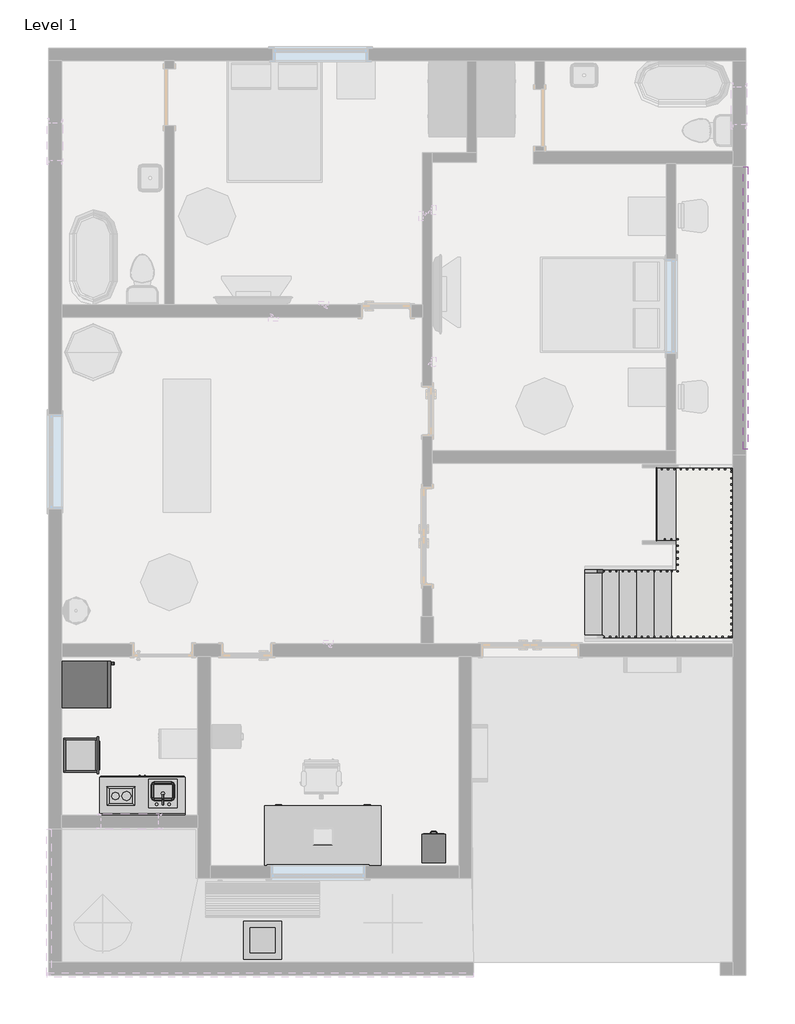
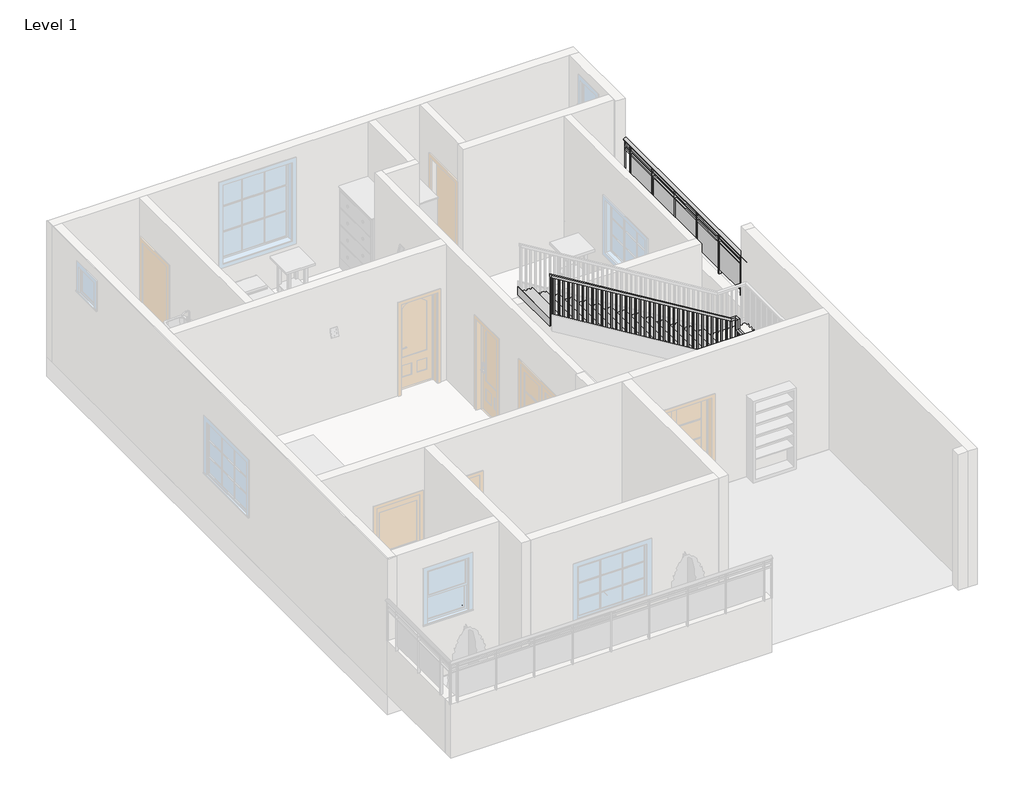
# One storey, part 3 of 4: 4 furniture elements, 4 proxies, 2 railings, 2 stair flights, 1 flow terminal, 1 slab.
"""IFC4 building model written with IfcOpenShell, lengths in millimetres."""

from ifc_helpers import new_model, si_unit, point, frame, origin, place, context, project, spatial, polyline, ellipse_curve, trimmed, outline, extrude, faceted_brep, transform, mapped, element, save
from ifc_brep_helpers import plane_surface, extruded_surface, advanced_brep
from components import proxy_fe84b772, proxy_844211aa, proxy_8b8c2dc4, proxy_a13a33b2, flow_terminal_871c2e40, furniture_d4d3357e, furniture_95afb093, furniture_2fc54265, furniture_b5c51a22, non_monolithic_landing_4509e35c, stair_flight_239b6ec8, stair_flight_7a186021

model = new_model("IFC4")

# Units and contexts
model_context = context("Model", 3, world=origin())
ifc_project = project(units=[si_unit("LENGTHUNIT", "METRE", prefix="MILLI")], contexts=[model_context])

# Site, building, storey
site = spatial("IfcSite", under=ifc_project)
building = spatial("IfcBuilding", under=site)
storey = spatial("IfcBuildingStorey", under=building, Name="Level 1", Elevation=0.0)

# Proxies
placement = place(None, origin())
proxy_shape = proxy_fe84b772(model_context)
element("IfcBuildingElementProxy", 1, Name="Cook Top-2 Unit : 12\" x 18\"", ObjectType="Cook Top-2 Unit : 12\" x 18\"", at=placement, inside=storey, context=model_context, shape_type="MappedRepresentation", body=[
    mapped(proxy_shape, transform((-10639.7134239, 21.3574946, 0.0), x_axis=(0.0, -1.0, 0.0), y_axis=(1.0, 0.0, 0.0), z_axis=(0.0, 0.0, 1.0))),
])
proxy_2_shape = proxy_844211aa(model_context)
element("IfcBuildingElementProxy", 2, Name="Kitchenette - Small : 54\"", ObjectType="Kitchenette - Small : 54\"", at=placement, inside=storey, context=model_context, shape_type="MappedRepresentation", body=[
    mapped(proxy_2_shape, transform((-10247.8509234, -359.6425054, 0.0), x_axis=(-1.0, 0.0, 0.0), y_axis=(0.0, -1.0, 0.0), z_axis=(0.0, 0.0, 1.0))),
])
proxy_3_shape = proxy_8b8c2dc4(model_context)
element("IfcBuildingElementProxy", 3, Name="Oven Double-Built-in : 21 1/2\" x 39 1/4\" x 21\"", ObjectType="Oven Double-Built-in : 21 1/2\" x 39 1/4\" x 21\"", at=placement, inside=storey, context=model_context, shape_type="MappedRepresentation", body=[
    mapped(proxy_3_shape, transform((-11116.1227694, 633.3465736, 0.0), x_axis=(0.0, 1.0, 0.0), y_axis=(-1.0, 0.0, 0.0), z_axis=(0.0, 0.0, 1.0))),
])
proxy_4_shape = proxy_a13a33b2(model_context)
element("IfcBuildingElementProxy", 4, Name="Refrigerator : 30\" x 32\" RH", ObjectType="Refrigerator : 30\" x 32\" RH", at=placement, inside=storey, context=model_context, shape_type="MappedRepresentation", body=[
    mapped(proxy_4_shape, transform((-11188.9261283, 1734.6585231, 0.0), x_axis=(0.0, 1.0000000000000002, 0.0), y_axis=(-1.0000000000000002, 0.0, 0.0), z_axis=(0.0, 0.0, 1.0))),
])

# Flow terminal
flow_terminal_shape = flow_terminal_871c2e40(model_context)
element("IfcFlowTerminal", 5, ObjectType="Sink Kitchen-Island : 18\" x 18\"", at=placement, inside=storey, context=model_context, shape_type="MappedRepresentation", body=[
    mapped(flow_terminal_shape, transform((-9920.6993877, -14.3971043, 0.0), x_axis=(-1.0, 0.0, 0.0), y_axis=(0.0, -1.0, 0.0), z_axis=(0.0, 0.0, 1.0))),
])

# Furniture
furniture_shape = furniture_d4d3357e(model_context)
element("IfcFurniture", 6, ObjectType="Cabinet-File 5 Drawer : 15\" x 18\"", at=placement, inside=storey, context=model_context, shape_type="MappedRepresentation", body=[
    mapped(furniture_shape, transform((-5720.8850753, -1035.1768056, 0.0), x_axis=(-1.0000000000000002, 0.0, 0.0), y_axis=(0.0, -1.0000000000000002, 0.0), z_axis=(0.0, 0.0, 1.0))),
])
furniture_2_shape = furniture_95afb093(model_context)
element("IfcFurniture", 7, ObjectType="Counter Top w Sink Hole : 24\" Depth", at=placement, inside=storey, context=model_context, shape_type="MappedRepresentation", body=[
    mapped(furniture_2_shape, transform((-10781.2509234, -359.6425054, 0.0), x_axis=(-1.0, 0.0, 0.0), y_axis=(0.0, -1.0, 0.0), z_axis=(0.0, 0.0, 1.0))),
])
furniture_3_shape = furniture_2fc54265(model_context)
element("IfcFurniture", 8, ObjectType="Desk : 72\" x 36\"", at=placement, inside=storey, context=model_context, shape_type="MappedRepresentation", body=[
    mapped(furniture_3_shape, transform((-8285.3886283, -1147.0425054, 0.0), x_axis=(1.0, 0.0, 0.0), y_axis=(0.0, 1.0, 0.0), z_axis=(0.0, 0.0, 1.0))),
])
furniture_4_shape = furniture_b5c51a22(model_context)
element("IfcFurniture", 9, ObjectType="Table-Coffee : 24\" x 24\" x 24\"", at=placement, inside=storey, context=model_context, shape_type="MappedRepresentation", body=[
    mapped(furniture_4_shape, transform((-8355.0107762, -2461.4535832, 0.0), x_axis=(1.0, 0.0, 0.0), y_axis=(0.0, 1.0, 0.0), z_axis=(0.0, 0.0, 1.0))),
])

# Railings
element("IfcRailing", 10, ObjectType="Glass Panel - Bottom Fill", at=placement, inside=storey, context=model_context, shape_type="SolidModel", body=[
    advanced_brep(
    [(-627.2886283, 5507.7574946, 2133.6), (-551.0886283, 5507.7574946, 2133.6), (-627.2886283, 10028.9574946, 2133.6), (-551.0886283, 10028.9574946, 2133.6)],
    [
        (0, 1, ellipse_curve(frame((-589.1886283, 5507.7574946, 2133.6), z_axis=(0.0, -1.0, 0.0), x_axis=(1.0, 0.0, 0.0)), 38.1, 28.575)),
        (1, 0, ellipse_curve(frame((-589.1886283, 5507.7574946, 2133.6), z_axis=(0.0, -1.0, 0.0), x_axis=(1.0, 0.0, 0.0)), 38.1, 28.575)),
        (2, 3, ellipse_curve(frame((-589.1886283, 10028.9574946, 2133.6), z_axis=(0.0, 1.0, 0.0), x_axis=(1.0, 0.0, 0.0)), 38.1, 28.575)),
        (3, 2, ellipse_curve(frame((-589.1886283, 10028.9574946, 2133.6), z_axis=(0.0, 1.0, 0.0), x_axis=(1.0, 0.0, 0.0)), 38.1, 28.575)),
        (0, 2),
        (3, 1),
    ],
    [
        plane_surface(frame((-589.1886283, 5507.7574946, 2133.6), z_axis=(0.0, -1.0, 0.0), x_axis=(0.0, 0.0, 1.0))),
        plane_surface(frame((-589.1886283, 10028.9574946, 2133.6), z_axis=(0.0, 1.0, 0.0), x_axis=(0.0, 0.0, 1.0))),
        extruded_surface(trimmed(ellipse_curve(frame((-589.1886283, 10028.9574946, 2133.6), z_axis=(0.0, -1.0, 0.0), x_axis=(1.0, 0.0, 0.0)), 38.1, 28.575), [point((-627.2886283, 10028.9574946, 2133.6))], [point((-551.0886283, 10028.9574946, 2133.6))], True, "CARTESIAN"), (0.0, -4521.199999999999, 0.0), 4521.199999999999),
        extruded_surface(trimmed(ellipse_curve(frame((-589.1886283, 10028.9574946, 2133.6), z_axis=(0.0, -1.0, 0.0), x_axis=(1.0, 0.0, 0.0)), 38.1, 28.575), [point((-551.0886283, 10028.9574946, 2133.6))], [point((-627.2886283, 10028.9574946, 2133.6))], True, "CARTESIAN"), (0.0, -4521.199999999999, 0.0), 4521.199999999999),
    ],
    [
        (0, [[1, 2]]),
        (1, [[3, 4]]),
        (2, [[-1, 5, -4, 6]]),
        (3, [[-2, -6, -3, -5]]),
    ],
),
    extrude(outline(polyline([(-576.4886283, 5507.7574946), (-601.8886283, 5507.7574946), (-601.8886283, 10028.9574946), (-576.4886283, 10028.9574946), (-576.4886283, 5507.7574946)])), frame((0.0, 0.0, 2019.3), z_axis=(0.0, 0.0, 1.0), x_axis=(1.0, 0.0, 0.0)), (0.0, 0.0, 1.0), 25.4),
    extrude(outline(polyline([(-576.4886283, 5507.7574946), (-601.8886283, 5507.7574946), (-601.8886283, 10028.9574946), (-576.4886283, 10028.9574946), (-576.4886283, 5507.7574946)])), frame((0.0, 0.0, 1917.7), z_axis=(0.0, 0.0, 1.0), x_axis=(1.0, 0.0, 0.0)), (0.0, 0.0, 1.0), 25.4),
    extrude(outline(polyline([(-563.7886283, 9794.0074946), (-614.5886283, 9794.0074946), (-614.5886283, 9806.7074946), (-563.7886283, 9806.7074946), (-563.7886283, 9794.0074946)])), frame((0.0, 0.0, 1219.2), z_axis=(0.0, 0.0, 1.0), x_axis=(1.0, 0.0, 0.0)), (0.0, 0.0, 1.0), 885.6788223),
    extrude(outline(polyline([(-595.7237853, 8987.5574946), (-595.7237853, 9800.3574946), (-589.3737853, 9800.3574946), (-589.3737853, 8987.5574946), (-595.7237853, 8987.5574946)])), frame((0.0, 0.0, 1320.8), z_axis=(0.0, 0.0, 1.0), x_axis=(1.0, 0.0, 0.0)), (0.0, 0.0, 1.0), 596.9),
    extrude(outline(polyline([(-563.7886283, 8981.2074946), (-614.5886283, 8981.2074946), (-614.5886283, 8993.9074946), (-563.7886283, 8993.9074946), (-563.7886283, 8981.2074946)])), frame((0.0, 0.0, 1219.2), z_axis=(0.0, 0.0, 1.0), x_axis=(1.0, 0.0, 0.0)), (0.0, 0.0, 1.0), 885.6788223),
    extrude(outline(polyline([(-595.7237853, 8174.7574946), (-595.7237853, 8987.5574946), (-589.3737853, 8987.5574946), (-589.3737853, 8174.7574946), (-595.7237853, 8174.7574946)])), frame((0.0, 0.0, 1320.8), z_axis=(0.0, 0.0, 1.0), x_axis=(1.0, 0.0, 0.0)), (0.0, 0.0, 1.0), 596.9),
    extrude(outline(polyline([(-563.7886283, 8168.4074946), (-614.5886283, 8168.4074946), (-614.5886283, 8181.1074946), (-563.7886283, 8181.1074946), (-563.7886283, 8168.4074946)])), frame((0.0, 0.0, 1219.2), z_axis=(0.0, 0.0, 1.0), x_axis=(1.0, 0.0, 0.0)), (0.0, 0.0, 1.0), 885.6788223),
    extrude(outline(polyline([(-595.7237853, 7361.9574946), (-595.7237853, 8174.7574946), (-589.3737853, 8174.7574946), (-589.3737853, 7361.9574946), (-595.7237853, 7361.9574946)])), frame((0.0, 0.0, 1320.8), z_axis=(0.0, 0.0, 1.0), x_axis=(1.0, 0.0, 0.0)), (0.0, 0.0, 1.0), 596.9),
    extrude(outline(polyline([(-563.7886283, 7355.6074946), (-614.5886283, 7355.6074946), (-614.5886283, 7368.3074946), (-563.7886283, 7368.3074946), (-563.7886283, 7355.6074946)])), frame((0.0, 0.0, 1219.2), z_axis=(0.0, 0.0, 1.0), x_axis=(1.0, 0.0, 0.0)), (0.0, 0.0, 1.0), 885.6788223),
    extrude(outline(polyline([(-595.7237853, 6549.1574946), (-595.7237853, 7361.9574946), (-589.3737853, 7361.9574946), (-589.3737853, 6549.1574946), (-595.7237853, 6549.1574946)])), frame((0.0, 0.0, 1320.8), z_axis=(0.0, 0.0, 1.0), x_axis=(1.0, 0.0, 0.0)), (0.0, 0.0, 1.0), 596.9),
    extrude(outline(polyline([(-563.7886283, 6542.8074946), (-614.5886283, 6542.8074946), (-614.5886283, 6555.5074946), (-563.7886283, 6555.5074946), (-563.7886283, 6542.8074946)])), frame((0.0, 0.0, 1219.2), z_axis=(0.0, 0.0, 1.0), x_axis=(1.0, 0.0, 0.0)), (0.0, 0.0, 1.0), 885.6788223),
    extrude(outline(polyline([(-595.7237853, 5736.3574946), (-595.7237853, 6549.1574946), (-589.3737853, 6549.1574946), (-589.3737853, 5736.3574946), (-595.7237853, 5736.3574946)])), frame((0.0, 0.0, 1320.8), z_axis=(0.0, 0.0, 1.0), x_axis=(1.0, 0.0, 0.0)), (0.0, 0.0, 1.0), 596.9),
    extrude(outline(polyline([(-563.7886283, 5730.0074946), (-614.5886283, 5730.0074946), (-614.5886283, 5742.7074946), (-563.7886283, 5742.7074946), (-563.7886283, 5730.0074946)])), frame((0.0, 0.0, 1219.2), z_axis=(0.0, 0.0, 1.0), x_axis=(1.0, 0.0, 0.0)), (0.0, 0.0, 1.0), 885.6788223),
    extrude(outline(polyline([(-579.6636283, 10016.2574946), (-598.7136283, 10016.2574946), (-598.7136283, 10035.3074946), (-579.6636283, 10035.3074946), (-579.6636283, 10016.2574946)])), frame((0.0, 0.0, 1219.2), z_axis=(0.0, 0.0, 1.0), x_axis=(1.0, 0.0, 0.0)), (0.0, 0.0, 1.0), 885.6788223),
    extrude(outline(polyline([(-579.6636283, 5501.4074946), (-598.7136283, 5501.4074946), (-598.7136283, 5520.4574946), (-579.6636283, 5520.4574946), (-579.6636283, 5501.4074946)])), frame((0.0, 0.0, 1219.2), z_axis=(0.0, 0.0, 1.0), x_axis=(1.0, 0.0, 0.0)), (0.0, 0.0, 1.0), 885.6788223),
])
element("IfcRailing", 11, ObjectType="Handrail - Rectangular", at=placement, inside=storey, context=model_context, shape_type="SolidModel", body=[
    faceted_brep([(-3170.5888787, 3576.1973029, 1083.7333333), (-3170.5888787, 3576.1973029, 1024.3318731), (-3170.5888787, 3525.3973029, 1024.3318731), (-3170.5888787, 3525.3973029, 1083.7333333), (-1773.5888787, 3576.1973029, 1930.4), (-1759.3964693, 3576.1973029, 1879.6), (-1759.3964693, 3525.3973029, 1879.6), (-1773.5888787, 3525.3973029, 1930.4), (-1706.7886283, 3576.1973029, 1930.4), (-1706.7886283, 3576.1973029, 1879.6), (-1655.9886283, 3525.3973029, 1879.6), (-1655.9886283, 3525.3973029, 1930.4), (-1706.7886283, 3958.3574946, 1930.4), (-1706.7886283, 4009.1574946, 1879.6), (-1655.9886283, 4009.1574946, 1879.6), (-1655.9886283, 3958.3574946, 1930.4), (-1706.7886283, 3958.3574946, 2145.9151515), (-1706.7886283, 4009.1574946, 2095.1151515), (-1655.9886283, 4009.1574946, 2095.1151515), (-1655.9886283, 3958.3574946, 2145.9151515), (-1706.7886283, 4034.5574946, 2145.9151515), (-1706.7886283, 4034.5574946, 2095.1151515), (-1655.9886283, 4085.3574946, 2095.1151515), (-1655.9886283, 4085.3574946, 2145.9151515), (-1782.9886283, 4034.5574946, 2145.9151515), (-1797.1810377, 4034.5574946, 2095.1151515), (-1797.1810377, 4085.3574946, 2095.1151515), (-1782.9886283, 4085.3574946, 2145.9151515), (-5618.3886283, 4034.5574946, 4470.4), (-5618.3886283, 4085.3574946, 4470.4), (-5618.3886283, 4085.3574946, 4410.9985397), (-5618.3886283, 4034.5574946, 4410.9985397)], [[[0, 1, 2, 3]], [[1, 0, 4, 5]], [[2, 1, 5, 6]], [[3, 2, 6, 7]], [[0, 3, 7, 4]], [[5, 4, 8, 9]], [[6, 5, 9, 10]], [[7, 6, 10, 11]], [[4, 7, 11, 8]], [[9, 8, 12, 13]], [[10, 9, 13, 14]], [[11, 10, 14, 15]], [[8, 11, 15, 12]], [[13, 12, 16, 17]], [[14, 13, 17, 18]], [[15, 14, 18, 19]], [[12, 15, 19, 16]], [[17, 16, 20, 21]], [[18, 17, 21, 22]], [[19, 18, 22, 23]], [[16, 19, 23, 20]], [[21, 20, 24, 25]], [[22, 21, 25, 26]], [[23, 22, 26, 27]], [[20, 23, 27, 24]], [[28, 29, 30, 31]], [[25, 24, 28, 31]], [[26, 25, 31, 30]], [[27, 26, 30, 29]], [[24, 27, 29, 28]]]),
    extrude(outline(polyline([(4370.5894488, -5551.7136283), (3386.6666667, -5551.7136283), (3386.6666667, -5532.6636283), (4359.0439943, -5532.6636283), (4370.5894488, -5551.7136283)])), frame((0.0, 4050.4324946, 0.0), z_axis=(0.0, 1.0, 0.0), x_axis=(0.0, 0.0, 1.0)), (0.0, 0.0, 1.0), 19.05),
    extrude(outline(polyline([(4309.0136913, -5450.1136283), (3386.6666667, -5450.1136283), (3386.6666667, -5431.0636283), (4297.4682367, -5431.0636283), (4309.0136913, -5450.1136283)])), frame((0.0, 4050.4324946, 0.0), z_axis=(0.0, 1.0, 0.0), x_axis=(0.0, 0.0, 1.0)), (0.0, 0.0, 1.0), 19.05),
    extrude(outline(polyline([(4247.4379337, -5348.5136283), (3386.6666667, -5348.5136283), (3386.6666667, -5329.4636283), (4235.8924791, -5329.4636283), (4247.4379337, -5348.5136283)])), frame((0.0, 4050.4324946, 0.0), z_axis=(0.0, 1.0, 0.0), x_axis=(0.0, 0.0, 1.0)), (0.0, 0.0, 1.0), 19.05),
    extrude(outline(polyline([(4185.8621761, -5246.9136283), (3217.3333333, -5246.9136283), (3217.3333333, -5227.8636283), (4174.3167216, -5227.8636283), (4185.8621761, -5246.9136283)])), frame((0.0, 4050.4324946, 0.0), z_axis=(0.0, 1.0, 0.0), x_axis=(0.0, 0.0, 1.0)), (0.0, 0.0, 1.0), 19.05),
    extrude(outline(polyline([(4124.2864185, -5145.3136283), (3217.3333333, -5145.3136283), (3217.3333333, -5126.2636283), (4112.740964, -5126.2636283), (4124.2864185, -5145.3136283)])), frame((0.0, 4050.4324946, 0.0), z_axis=(0.0, 1.0, 0.0), x_axis=(0.0, 0.0, 1.0)), (0.0, 0.0, 1.0), 19.05),
    extrude(outline(polyline([(4062.710661, -5043.7136283), (3048.0, -5043.7136283), (3048.0, -5024.6636283), (4051.1652064, -5024.6636283), (4062.710661, -5043.7136283)])), frame((0.0, 4050.4324946, 0.0), z_axis=(0.0, 1.0, 0.0), x_axis=(0.0, 0.0, 1.0)), (0.0, 0.0, 1.0), 19.05),
    extrude(outline(polyline([(4001.1349034, -4942.1136283), (3048.0, -4942.1136283), (3048.0, -4923.0636283), (3989.5894488, -4923.0636283), (4001.1349034, -4942.1136283)])), frame((0.0, 4050.4324946, 0.0), z_axis=(0.0, 1.0, 0.0), x_axis=(0.0, 0.0, 1.0)), (0.0, 0.0, 1.0), 19.05),
    extrude(outline(polyline([(3939.5591458, -4840.5136283), (3048.0, -4840.5136283), (3048.0, -4821.4636283), (3928.0136913, -4821.4636283), (3939.5591458, -4840.5136283)])), frame((0.0, 4050.4324946, 0.0), z_axis=(0.0, 1.0, 0.0), x_axis=(0.0, 0.0, 1.0)), (0.0, 0.0, 1.0), 19.05),
    extrude(outline(polyline([(3877.9833882, -4738.9136283), (2878.6666667, -4738.9136283), (2878.6666667, -4719.8636283), (3866.4379337, -4719.8636283), (3877.9833882, -4738.9136283)])), frame((0.0, 4050.4324946, 0.0), z_axis=(0.0, 1.0, 0.0), x_axis=(0.0, 0.0, 1.0)), (0.0, 0.0, 1.0), 19.05),
    extrude(outline(polyline([(3816.4076307, -4637.3136283), (2878.6666667, -4637.3136283), (2878.6666667, -4618.2636283), (3804.8621761, -4618.2636283), (3816.4076307, -4637.3136283)])), frame((0.0, 4050.4324946, 0.0), z_axis=(0.0, 1.0, 0.0), x_axis=(0.0, 0.0, 1.0)), (0.0, 0.0, 1.0), 19.05),
    extrude(outline(polyline([(3754.8318731, -4535.7136283), (2878.6666667, -4535.7136283), (2878.6666667, -4516.6636283), (3743.2864185, -4516.6636283), (3754.8318731, -4535.7136283)])), frame((0.0, 4050.4324946, 0.0), z_axis=(0.0, 1.0, 0.0), x_axis=(0.0, 0.0, 1.0)), (0.0, 0.0, 1.0), 19.05),
    extrude(outline(polyline([(3693.2561155, -4434.1136283), (2709.3333333, -4434.1136283), (2709.3333333, -4415.0636283), (3681.710661, -4415.0636283), (3693.2561155, -4434.1136283)])), frame((0.0, 4050.4324946, 0.0), z_axis=(0.0, 1.0, 0.0), x_axis=(0.0, 0.0, 1.0)), (0.0, 0.0, 1.0), 19.05),
    extrude(outline(polyline([(3631.6803579, -4332.5136283), (2709.3333333, -4332.5136283), (2709.3333333, -4313.4636283), (3620.1349034, -4313.4636283), (3631.6803579, -4332.5136283)])), frame((0.0, 4050.4324946, 0.0), z_axis=(0.0, 1.0, 0.0), x_axis=(0.0, 0.0, 1.0)), (0.0, 0.0, 1.0), 19.05),
    extrude(outline(polyline([(3570.1046004, -4230.9136283), (2709.3333333, -4230.9136283), (2709.3333333, -4211.8636283), (3558.5591458, -4211.8636283), (3570.1046004, -4230.9136283)])), frame((0.0, 4050.4324946, 0.0), z_axis=(0.0, 1.0, 0.0), x_axis=(0.0, 0.0, 1.0)), (0.0, 0.0, 1.0), 19.05),
    extrude(outline(polyline([(3508.5288428, -4129.3136283), (2540.0, -4129.3136283), (2540.0, -4110.2636283), (3496.9833882, -4110.2636283), (3508.5288428, -4129.3136283)])), frame((0.0, 4050.4324946, 0.0), z_axis=(0.0, 1.0, 0.0), x_axis=(0.0, 0.0, 1.0)), (0.0, 0.0, 1.0), 19.05),
    extrude(outline(polyline([(3446.9530852, -4027.7136283), (2540.0, -4027.7136283), (2540.0, -4008.6636283), (3435.4076307, -4008.6636283), (3446.9530852, -4027.7136283)])), frame((0.0, 4050.4324946, 0.0), z_axis=(0.0, 1.0, 0.0), x_axis=(0.0, 0.0, 1.0)), (0.0, 0.0, 1.0), 19.05),
    extrude(outline(polyline([(3385.3773276, -3926.1136283), (2370.6666667, -3926.1136283), (2370.6666667, -3907.0636283), (3373.8318731, -3907.0636283), (3385.3773276, -3926.1136283)])), frame((0.0, 4050.4324946, 0.0), z_axis=(0.0, 1.0, 0.0), x_axis=(0.0, 0.0, 1.0)), (0.0, 0.0, 1.0), 19.05),
    extrude(outline(polyline([(3323.80157, -3824.5136283), (2370.6666667, -3824.5136283), (2370.6666667, -3805.4636283), (3312.2561155, -3805.4636283), (3323.80157, -3824.5136283)])), frame((0.0, 4050.4324946, 0.0), z_axis=(0.0, 1.0, 0.0), x_axis=(0.0, 0.0, 1.0)), (0.0, 0.0, 1.0), 19.05),
    extrude(outline(polyline([(3262.2258125, -3722.9136283), (2370.6666667, -3722.9136283), (2370.6666667, -3703.8636283), (3250.6803579, -3703.8636283), (3262.2258125, -3722.9136283)])), frame((0.0, 4050.4324946, 0.0), z_axis=(0.0, 1.0, 0.0), x_axis=(0.0, 0.0, 1.0)), (0.0, 0.0, 1.0), 19.05),
    extrude(outline(polyline([(3200.6500549, -3621.3136283), (2201.3333333, -3621.3136283), (2201.3333333, -3602.2636283), (3189.1046004, -3602.2636283), (3200.6500549, -3621.3136283)])), frame((0.0, 4050.4324946, 0.0), z_axis=(0.0, 1.0, 0.0), x_axis=(0.0, 0.0, 1.0)), (0.0, 0.0, 1.0), 19.05),
    extrude(outline(polyline([(3139.0742973, -3519.7136283), (2201.3333333, -3519.7136283), (2201.3333333, -3500.6636283), (3127.5288428, -3500.6636283), (3139.0742973, -3519.7136283)])), frame((0.0, 4050.4324946, 0.0), z_axis=(0.0, 1.0, 0.0), x_axis=(0.0, 0.0, 1.0)), (0.0, 0.0, 1.0), 19.05),
    extrude(outline(polyline([(3077.4985397, -3418.1136283), (2201.3333333, -3418.1136283), (2201.3333333, -3399.0636283), (3065.9530852, -3399.0636283), (3077.4985397, -3418.1136283)])), frame((0.0, 4050.4324946, 0.0), z_axis=(0.0, 1.0, 0.0), x_axis=(0.0, 0.0, 1.0)), (0.0, 0.0, 1.0), 19.05),
    extrude(outline(polyline([(3015.9227822, -3316.5136283), (2032.0, -3316.5136283), (2032.0, -3297.4636283), (3004.3773276, -3297.4636283), (3015.9227822, -3316.5136283)])), frame((0.0, 4050.4324946, 0.0), z_axis=(0.0, 1.0, 0.0), x_axis=(0.0, 0.0, 1.0)), (0.0, 0.0, 1.0), 19.05),
    extrude(outline(polyline([(2954.3470246, -3214.9136283), (2032.0, -3214.9136283), (2032.0, -3195.8636283), (2942.80157, -3195.8636283), (2954.3470246, -3214.9136283)])), frame((0.0, 4050.4324946, 0.0), z_axis=(0.0, 1.0, 0.0), x_axis=(0.0, 0.0, 1.0)), (0.0, 0.0, 1.0), 19.05),
    extrude(outline(polyline([(2892.771267, -3113.3136283), (2032.0, -3113.3136283), (2032.0, -3094.2636283), (2881.2258125, -3094.2636283), (2892.771267, -3113.3136283)])), frame((0.0, 4050.4324946, 0.0), z_axis=(0.0, 1.0, 0.0), x_axis=(0.0, 0.0, 1.0)), (0.0, 0.0, 1.0), 19.05),
    extrude(outline(polyline([(2831.1955094, -3011.7136283), (1862.6666667, -3011.7136283), (1862.6666667, -2992.6636283), (2819.6500549, -2992.6636283), (2831.1955094, -3011.7136283)])), frame((0.0, 4050.4324946, 0.0), z_axis=(0.0, 1.0, 0.0), x_axis=(0.0, 0.0, 1.0)), (0.0, 0.0, 1.0), 19.05),
    extrude(outline(polyline([(2769.6197519, -2910.1136283), (1862.6666667, -2910.1136283), (1862.6666667, -2891.0636283), (2758.0742973, -2891.0636283), (2769.6197519, -2910.1136283)])), frame((0.0, 4050.4324946, 0.0), z_axis=(0.0, 1.0, 0.0), x_axis=(0.0, 0.0, 1.0)), (0.0, 0.0, 1.0), 19.05),
    extrude(outline(polyline([(2708.0439943, -2808.5136283), (1693.3333333, -2808.5136283), (1693.3333333, -2789.4636283), (2696.4985397, -2789.4636283), (2708.0439943, -2808.5136283)])), frame((0.0, 4050.4324946, 0.0), z_axis=(0.0, 1.0, 0.0), x_axis=(0.0, 0.0, 1.0)), (0.0, 0.0, 1.0), 19.05),
    extrude(outline(polyline([(2646.4682367, -2706.9136283), (1693.3333333, -2706.9136283), (1693.3333333, -2687.8636283), (2634.9227822, -2687.8636283), (2646.4682367, -2706.9136283)])), frame((0.0, 4050.4324946, 0.0), z_axis=(0.0, 1.0, 0.0), x_axis=(0.0, 0.0, 1.0)), (0.0, 0.0, 1.0), 19.05),
    extrude(outline(polyline([(2584.8924791, -2605.3136283), (1693.3333333, -2605.3136283), (1693.3333333, -2586.2636283), (2573.3470246, -2586.2636283), (2584.8924791, -2605.3136283)])), frame((0.0, 4050.4324946, 0.0), z_axis=(0.0, 1.0, 0.0), x_axis=(0.0, 0.0, 1.0)), (0.0, 0.0, 1.0), 19.05),
    extrude(outline(polyline([(2523.3167216, -2503.7136283), (1524.0, -2503.7136283), (1524.0, -2484.6636283), (2511.771267, -2484.6636283), (2523.3167216, -2503.7136283)])), frame((0.0, 4050.4324946, 0.0), z_axis=(0.0, 1.0, 0.0), x_axis=(0.0, 0.0, 1.0)), (0.0, 0.0, 1.0), 19.05),
    extrude(outline(polyline([(2461.740964, -2402.1136283), (1524.0, -2402.1136283), (1524.0, -2383.0636283), (2450.1955094, -2383.0636283), (2461.740964, -2402.1136283)])), frame((0.0, 4050.4324946, 0.0), z_axis=(0.0, 1.0, 0.0), x_axis=(0.0, 0.0, 1.0)), (0.0, 0.0, 1.0), 19.05),
    extrude(outline(polyline([(2400.1652064, -2300.5136283), (1524.0, -2300.5136283), (1524.0, -2281.4636283), (2388.6197519, -2281.4636283), (2400.1652064, -2300.5136283)])), frame((0.0, 4050.4324946, 0.0), z_axis=(0.0, 1.0, 0.0), x_axis=(0.0, 0.0, 1.0)), (0.0, 0.0, 1.0), 19.05),
    extrude(outline(polyline([(2338.5894488, -2198.9136283), (1354.6666667, -2198.9136283), (1354.6666667, -2179.8636283), (2327.0439943, -2179.8636283), (2338.5894488, -2198.9136283)])), frame((0.0, 4050.4324946, 0.0), z_axis=(0.0, 1.0, 0.0), x_axis=(0.0, 0.0, 1.0)), (0.0, 0.0, 1.0), 19.05),
    extrude(outline(polyline([(2277.0136913, -2097.3136283), (1354.6666667, -2097.3136283), (1354.6666667, -2078.2636283), (2265.4682367, -2078.2636283), (2277.0136913, -2097.3136283)])), frame((0.0, 4050.4324946, 0.0), z_axis=(0.0, 1.0, 0.0), x_axis=(0.0, 0.0, 1.0)), (0.0, 0.0, 1.0), 19.05),
    extrude(outline(polyline([(2215.4379337, -1995.7136283), (1354.6666667, -1995.7136283), (1354.6666667, -1976.6636283), (2203.8924791, -1976.6636283), (2215.4379337, -1995.7136283)])), frame((0.0, 4050.4324946, 0.0), z_axis=(0.0, 1.0, 0.0), x_axis=(0.0, 0.0, 1.0)), (0.0, 0.0, 1.0), 19.05),
    extrude(outline(polyline([(2153.8621761, -1894.1136283), (1185.3333333, -1894.1136283), (1185.3333333, -1875.0636283), (2142.3167216, -1875.0636283), (2153.8621761, -1894.1136283)])), frame((0.0, 4050.4324946, 0.0), z_axis=(0.0, 1.0, 0.0), x_axis=(0.0, 0.0, 1.0)), (0.0, 0.0, 1.0), 19.05),
    extrude(outline(polyline([(-1773.4636283, 4050.4324946), (-1792.5136283, 4050.4324946), (-1792.5136283, 4069.4824946), (-1773.4636283, 4069.4824946), (-1773.4636283, 4050.4324946)])), frame((0.0, 0.0, 1185.3333333), z_axis=(0.0, 0.0, 1.0), x_axis=(1.0, 0.0, 0.0)), (0.0, 0.0, 1.0), 909.7818182),
    extrude(outline(polyline([(-1690.9136283, 4049.2723029), (-1690.9136283, 4068.3223029), (-1671.8636283, 4068.3223029), (-1671.8636283, 4049.2723029), (-1690.9136283, 4049.2723029)])), frame((0.0, 0.0, 1016.0), z_axis=(0.0, 0.0, 1.0), x_axis=(1.0, 0.0, 0.0)), (0.0, 0.0, 1.0), 1079.1151515),
    extrude(outline(polyline([(-1690.9136283, 3947.6723029), (-1690.9136283, 3966.7223029), (-1671.8636283, 3966.7223029), (-1671.8636283, 3947.6723029), (-1690.9136283, 3947.6723029)])), frame((0.0, 0.0, 1016.0), z_axis=(0.0, 0.0, 1.0), x_axis=(1.0, 0.0, 0.0)), (0.0, 0.0, 1.0), 863.6),
    extrude(outline(polyline([(-1690.9136283, 3846.0723029), (-1690.9136283, 3865.1223029), (-1671.8636283, 3865.1223029), (-1671.8636283, 3846.0723029), (-1690.9136283, 3846.0723029)])), frame((0.0, 0.0, 1016.0), z_axis=(0.0, 0.0, 1.0), x_axis=(1.0, 0.0, 0.0)), (0.0, 0.0, 1.0), 863.6),
    extrude(outline(polyline([(-1690.9136283, 3744.4723029), (-1690.9136283, 3763.5223029), (-1671.8636283, 3763.5223029), (-1671.8636283, 3744.4723029), (-1690.9136283, 3744.4723029)])), frame((0.0, 0.0, 1016.0), z_axis=(0.0, 0.0, 1.0), x_axis=(1.0, 0.0, 0.0)), (0.0, 0.0, 1.0), 863.6),
    extrude(outline(polyline([(-1690.9136283, 3642.8723029), (-1690.9136283, 3661.9223029), (-1671.8636283, 3661.9223029), (-1671.8636283, 3642.8723029), (-1690.9136283, 3642.8723029)])), frame((0.0, 0.0, 1016.0), z_axis=(0.0, 0.0, 1.0), x_axis=(1.0, 0.0, 0.0)), (0.0, 0.0, 1.0), 863.6),
    extrude(outline(polyline([(1819.0439943, -1859.3138787), (846.6666667, -1859.3138787), (846.6666667, -1840.2638787), (1830.5894488, -1840.2638787), (1819.0439943, -1859.3138787)])), frame((0.0, 3541.2723029, 0.0), z_axis=(0.0, 1.0, 0.0), x_axis=(0.0, 0.0, 1.0)), (0.0, 0.0, 1.0), 19.05),
    extrude(outline(polyline([(1757.4682367, -1960.9138787), (846.6666667, -1960.9138787), (846.6666667, -1941.8638787), (1769.0136913, -1941.8638787), (1757.4682367, -1960.9138787)])), frame((0.0, 3541.2723029, 0.0), z_axis=(0.0, 1.0, 0.0), x_axis=(0.0, 0.0, 1.0)), (0.0, 0.0, 1.0), 19.05),
    extrude(outline(polyline([(1695.8924791, -2062.5138787), (846.6666667, -2062.5138787), (846.6666667, -2043.4638787), (1707.4379337, -2043.4638787), (1695.8924791, -2062.5138787)])), frame((0.0, 3541.2723029, 0.0), z_axis=(0.0, 1.0, 0.0), x_axis=(0.0, 0.0, 1.0)), (0.0, 0.0, 1.0), 19.05),
    extrude(outline(polyline([(1634.3167216, -2164.1138787), (677.3333333, -2164.1138787), (677.3333333, -2145.0638787), (1645.8621761, -2145.0638787), (1634.3167216, -2164.1138787)])), frame((0.0, 3541.2723029, 0.0), z_axis=(0.0, 1.0, 0.0), x_axis=(0.0, 0.0, 1.0)), (0.0, 0.0, 1.0), 19.05),
    extrude(outline(polyline([(1572.740964, -2265.7138787), (677.3333333, -2265.7138787), (677.3333333, -2246.6638787), (1584.2864185, -2246.6638787), (1572.740964, -2265.7138787)])), frame((0.0, 3541.2723029, 0.0), z_axis=(0.0, 1.0, 0.0), x_axis=(0.0, 0.0, 1.0)), (0.0, 0.0, 1.0), 19.05),
    extrude(outline(polyline([(1511.1652064, -2367.3138787), (508.0, -2367.3138787), (508.0, -2348.2638787), (1522.710661, -2348.2638787), (1511.1652064, -2367.3138787)])), frame((0.0, 3541.2723029, 0.0), z_axis=(0.0, 1.0, 0.0), x_axis=(0.0, 0.0, 1.0)), (0.0, 0.0, 1.0), 19.05),
    extrude(outline(polyline([(1449.5894488, -2468.9138787), (508.0, -2468.9138787), (508.0, -2449.8638787), (1461.1349034, -2449.8638787), (1449.5894488, -2468.9138787)])), frame((0.0, 3541.2723029, 0.0), z_axis=(0.0, 1.0, 0.0), x_axis=(0.0, 0.0, 1.0)), (0.0, 0.0, 1.0), 19.05),
    extrude(outline(polyline([(1388.0136913, -2570.5138787), (508.0, -2570.5138787), (508.0, -2551.4638787), (1399.5591458, -2551.4638787), (1388.0136913, -2570.5138787)])), frame((0.0, 3541.2723029, 0.0), z_axis=(0.0, 1.0, 0.0), x_axis=(0.0, 0.0, 1.0)), (0.0, 0.0, 1.0), 19.05),
    extrude(outline(polyline([(1326.4379337, -2672.1138787), (338.6666667, -2672.1138787), (338.6666667, -2653.0638787), (1337.9833882, -2653.0638787), (1326.4379337, -2672.1138787)])), frame((0.0, 3541.2723029, 0.0), z_axis=(0.0, 1.0, 0.0), x_axis=(0.0, 0.0, 1.0)), (0.0, 0.0, 1.0), 19.05),
    extrude(outline(polyline([(1264.8621761, -2773.7138787), (338.6666667, -2773.7138787), (338.6666667, -2754.6638787), (1276.4076307, -2754.6638787), (1264.8621761, -2773.7138787)])), frame((0.0, 3541.2723029, 0.0), z_axis=(0.0, 1.0, 0.0), x_axis=(0.0, 0.0, 1.0)), (0.0, 0.0, 1.0), 19.05),
    extrude(outline(polyline([(1203.2864185, -2875.3138787), (338.6666667, -2875.3138787), (338.6666667, -2856.2638787), (1214.8318731, -2856.2638787), (1203.2864185, -2875.3138787)])), frame((0.0, 3541.2723029, 0.0), z_axis=(0.0, 1.0, 0.0), x_axis=(0.0, 0.0, 1.0)), (0.0, 0.0, 1.0), 19.05),
    extrude(outline(polyline([(1141.710661, -2976.9138787), (169.3333333, -2976.9138787), (169.3333333, -2957.8638787), (1153.2561155, -2957.8638787), (1141.710661, -2976.9138787)])), frame((0.0, 3541.2723029, 0.0), z_axis=(0.0, 1.0, 0.0), x_axis=(0.0, 0.0, 1.0)), (0.0, 0.0, 1.0), 19.05),
    extrude(outline(polyline([(1080.1349034, -3078.5138787), (169.3333333, -3078.5138787), (169.3333333, -3059.4638787), (1091.6803579, -3059.4638787), (1080.1349034, -3078.5138787)])), frame((0.0, 3541.2723029, 0.0), z_axis=(0.0, 1.0, 0.0), x_axis=(0.0, 0.0, 1.0)), (0.0, 0.0, 1.0), 19.05),
    extrude(outline(polyline([(-1671.8636283, 4050.4324946), (-1690.9136283, 4050.4324946), (-1690.9136283, 4069.4824946), (-1671.8636283, 4069.4824946), (-1671.8636283, 4050.4324946)])), frame((0.0, 0.0, 1016.0), z_axis=(0.0, 0.0, 1.0), x_axis=(1.0, 0.0, 0.0)), (0.0, 0.0, 1.0), 1079.1151515),
    extrude(outline(polyline([(-1690.9136283, 3560.3223029), (-1671.8636283, 3560.3223029), (-1671.8636283, 3541.2723029), (-1690.9136283, 3541.2723029), (-1690.9136283, 3560.3223029)])), frame((0.0, 0.0, 1016.0), z_axis=(0.0, 0.0, 1.0), x_axis=(1.0, 0.0, 0.0)), (0.0, 0.0, 1.0), 863.6),
    extrude(outline(polyline([(-1783.1138787, 3560.3223029), (-1764.0638787, 3560.3223029), (-1764.0638787, 3541.2723029), (-1783.1138787, 3541.2723029), (-1783.1138787, 3560.3223029)])), frame((0.0, 0.0, 1016.0), z_axis=(0.0, 0.0, 1.0), x_axis=(1.0, 0.0, 0.0)), (0.0, 0.0, 1.0), 863.6),
    extrude(outline(polyline([(4410.9985397, -5618.3886283), (3386.6666667, -5618.3886283), (3386.6666667, -5599.3386283), (4399.4530852, -5599.3386283), (4410.9985397, -5618.3886283)])), frame((0.0, 4050.4324946, 0.0), z_axis=(0.0, 1.0, 0.0), x_axis=(0.0, 0.0, 1.0)), (0.0, 0.0, 1.0), 19.05),
    extrude(outline(polyline([(1024.3318731, -3170.5888787), (169.3333333, -3170.5888787), (169.3333333, -3151.5388787), (1035.8773276, -3151.5388787), (1024.3318731, -3170.5888787)])), frame((0.0, 3541.2723029, 0.0), z_axis=(0.0, 1.0, 0.0), x_axis=(0.0, 0.0, 1.0)), (0.0, 0.0, 1.0), 19.05),
])

# Slab
non_monolithic_landing_shape = non_monolithic_landing_4509e35c(model_context)
element("IfcSlab", 12, ObjectType="Non-Monolithic Landing", at=placement, inside=storey, context=model_context, shape_type="MappedRepresentation", body=[
    mapped(non_monolithic_landing_shape, transform((0.0, 0.0, 0.0), x_axis=(1.0, 0.0, 0.0), y_axis=(0.0, 1.0, 0.0), z_axis=(0.0, 0.0, 1.0))),
])

# Stair flights
stair_flight_shape = stair_flight_239b6ec8(model_context)
element("IfcStairFlight", 13, ObjectType="2\" Tread 1\" Nosing 1/4\" Riser", at=placement, inside=storey, context=model_context, shape_type="MappedRepresentation", body=[
    mapped(stair_flight_shape, transform((0.0, 0.0, 0.0), x_axis=(1.0, 0.0, 0.0), y_axis=(0.0, 1.0, 0.0), z_axis=(0.0, 0.0, 1.0))),
])
stair_flight_2_shape = stair_flight_7a186021(model_context)
element("IfcStairFlight", 14, ObjectType="2\" Tread 1\" Nosing 1/4\" Riser", at=placement, inside=storey, context=model_context, shape_type="MappedRepresentation", body=[
    mapped(stair_flight_2_shape, transform((0.0, 0.0, 0.0), x_axis=(1.0, 0.0, 0.0), y_axis=(0.0, 1.0, 0.0), z_axis=(0.0, 0.0, 1.0))),
])

save(model, "model.ifc")

# Revit data of these elements
# Type "Cook Top-2 Unit : 12\" x 18\""
#   Assembly Code = "E1090400"
#   Counter Height = 3' - 0"
#   Depth = 1' - 6"
#   Width = 1' - 0"
#   Burner Material = Steel, Chrome Plated
#   Cooktop Material = Steel, Polished
#   Default Elevation = 0
# Type "Kitchenette - Small : 54\""
#   Assembly Code = "E1090400"
#   Width = 4' - 6"
#   Height = 2' - 10 1/2"
#   Depth = 2' - 0"
#   Toe Depth = 0' - 3"
#   Toe Height = 0' - 3 1/2"
#   Cabinet Material = Cabinets
#   Door/Drawer Material = Cabinets
#   Handle Material = Cabinets - Handles
#   Default Elevation = 0
# Type "Oven Double-Built-in : 21 1/2\" x 39 1/4\" x 21\""
#   Label = "OVEN"
#   Assembly Code = "E1090400"
#   Depth = 1' - 9"
#   Height = 3' - 3 1/4"
#   Width = 1' - 9 1/2"
#   Oven Material = Metal - Stainless Steel, Polished
#   Default Elevation = 0
# Type "Refrigerator : 30\" x 32\" RH"
#   Label = "REF."
#   Assembly Code = "E1090400"
#   Depth = 2' - 7 3/4"
#   Handle = 2' - 3"
#   Height = 5' - 10"
#   Rear Clearance = 0' - 2"
#   Top Door Height = 1' - 8"
#   Width = 2' - 5 3/8"
#   Material = Steel, Paint Finish, Ivory, Glossy
#   Default Elevation = 0
# Type "Sink Kitchen-Island : 18\" x 18\""
#   Assembly Code = "D2010410"
#   Counter Height = 3' - 0"
#   Depth = 1' - 6"
#   Width = 1' - 6"
#   Faucet Material = Steel, Polished
#   Sink Material = Steel, Polished
#   Default Elevation = 0
# Type "Cabinet-File 5 Drawer : 15\" x 18\""
#   Assembly Code = "E2020200"
#   Depth = 1' - 6"
#   Height = 5' - 0"
#   Width = 1' - 3"
#   Cabinet Material = Steel, Paint Finish, Ivory, Glossy
#   Handle Material = Steel, Chrome Plated
#   Default Elevation = 0
# Type "Counter Top w Sink Hole : 24\" Depth"
#   Assembly Code = "C1030400"
#   Counter Thickness = 0' - 1 1/2"
#   Depth [instance default] = 2' - 1"
#   Height = 3' - 0"
#   Length [instance default] = 8' - 0"
#   Sink Location [instance default] = 2' - 0"
#   Sink Location To Wall [instance default] = 0' - 6"
#   Sink Opening Depth [instance default] = 1' - 3"
#   Sink Opening Width [instance default] = 2' - 3"
#   Counter Top Material = none
#   Default Elevation = 0
# Type "Desk : 72\" x 36\""
#   Assembly Code = "E2020200"
#   Depth = 3' - 0"
#   Height = 2' - 6"
#   Leg Height = 0' - 6"
#   Width = 6' - 0"
#   Body Material = Laminate, Ivory, Matte
#   Handle/Leg Material = Steel, Chrome Plated
#   Top Material = Cherry
#   Default Elevation = 0
# Type "Table-Coffee : 24\" x 24\" x 24\""
#   Assembly Code = "E2020200"
#   Height = 2' - 0"
#   Length = 2' - 0"
#   Width = 2' - 0"
#   Top Material = none
#   Frame Material = none
#   Default Elevation = 0
# Type "Glass Panel - Bottom Fill"
#   Assembly Code = "C2010400"
#   built-in parameter 1008612 = 0.0416667 (stored number, unit not read)
#   built-in parameter 1008611 = 0.0416667 (stored number, unit not read)
#   built-in parameter 1008609 = 0.333333 (stored number, unit not read)
#   built-in parameter 1008604 = 0.166667 (stored number, unit not read)
#   built-in parameter 1008603 = 0.166667 (stored number, unit not read)
#   Railing Height = 3' - 0"
#   built-in parameter 1008630 = 2
#   built-in parameter 1008610 = 2
#   built-in parameter 1008618 = Baluster - Square : 3/4"
# Type "Handrail - Rectangular"
#   Assembly Code = "C2010400"
#   built-in parameter 1008612 = 0.0416667 (stored number, unit not read)
#   built-in parameter 1008611 = 0.0416667 (stored number, unit not read)
#   built-in parameter 1008609 = 0.333333 (stored number, unit not read)
#   built-in parameter 1008604 = 0.166667 (stored number, unit not read)
#   built-in parameter 1008603 = 0.166667 (stored number, unit not read)
#   Railing Height = 3' - 0"
#   built-in parameter 1008630 = 2
#   built-in parameter 1008610 = 2
#   built-in parameter 1008618 = Baluster - Square : 3/4"
# Element 1 (IfcBuildingElementProxy, "Cook Top-2 Unit : 12\" x 18\"")
#   Phase Created = New Construction
#   Materials on its faces: "Steel, Chrome Plated", "Steel, Polished"
# Element 2 (IfcBuildingElementProxy, "Kitchenette - Small : 54\"")
#   Phase Created = New Construction
#   Materials on its faces: "Cabinets", "Cabinets - Handles"
# Element 3 (IfcBuildingElementProxy, "Oven Double-Built-in : 21 1/2\" x 39 1/4\" x 21\"")
#   Phase Created = New Construction
#   Materials on its faces: "Steel", "Metal - Stainless Steel, Polished", "Glass"
# Element 4 (IfcBuildingElementProxy, "Refrigerator : 30\" x 32\" RH")
#   Phase Created = New Construction
#   Materials on its faces: "Steel, Paint Finish, Ivory, Glossy", "Steel, Chrome Plated"
# Element 5 (IfcFlowTerminal, "Sink Kitchen-Island : 18\" x 18\"")
#   Mark = "7"
#   Phase Created = New Construction
#   Materials on its faces: "Steel, Polished"
# Element 6 (IfcFurniture, "Cabinet-File 5 Drawer : 15\" x 18\"")
#   Phase Created = New Construction
#   Materials on its faces: "Steel, Chrome Plated", "Steel, Paint Finish, Ivory, Glossy"
# Element 7 (IfcFurniture, "Counter Top w Sink Hole : 24\" Depth")
#   Sink Opening Depth = 1' - 3"
#   Sink Location To Wall = 0' - 6"
#   Length = 4' - 6"
#   Sink Location = 1' - 2"
#   Sink Opening Width = 1' - 4"
#   Depth = 2' - 0"
#   Phase Created = New Construction
#   Materials on its faces: "Counter Top"
# Element 8 (IfcFurniture, "Desk : 72\" x 36\"")
#   Phase Created = New Construction
#   Materials on its faces: "Steel, Chrome Plated", "Laminate, Ivory, Matte", "Cherry"
# Element 9 (IfcFurniture, "Table-Coffee : 24\" x 24\" x 24\"")
#   Phase Created = New Construction
#   Materials on its faces: "Glass - Clear, Grey"
# Element 10 (IfcRailing, "Glass Panel - Bottom Fill")
#   built-in parameter 1008621 = 4 (stored number, unit not read)
#   Phase Created = New Construction
#   Materials on its faces: "Glass"
# Element 11 (IfcRailing, "Handrail - Rectangular")
#   Phase Created = New Construction
# Element 12 (IfcSlab, "Non-Monolithic Landing")
#   Phase Created = New Construction
# Elements 13, 14 (IfcStairFlight, "2\" Tread 1\" Nosing 1/4\" Riser")
#   Phase Created = New Construction
# Materials
#   "Steel, Chrome Plated": class "Metal", colour RGB 17 17 17, transparency 0, Description = "Chromiuim plated steel", Cost = 0
#   "Steel, Polished": class "Metal", colour RGB 57 57 57, transparency 0, Description = "Polished steel", Cost = 0
#   "Cabinets": colour RGB 249 249 249, transparency 0
#   "Cabinets - Handles": class "Metal", colour RGB 57 57 57, transparency 0
#   "Metal - Stainless Steel, Polished": class "Metal", colour RGB 216 216 216, transparency 0
#   "Steel, Paint Finish, Ivory, Glossy": class "Metal", colour RGB 247 247 239, transparency 0, Description = "Steel, paint finish, ivory, glossy", Cost = 0
#   "Laminate, Ivory, Matte": class "Plastic", colour RGB 247 247 239, transparency 0, Description = "Plastic Laminate - Ivory, Matte", Cost = 0
#   "Cherry": class "Wood", colour RGB 226 177 128, transparency 0, Description = "Prunus Serotina", Cost = 0
#   "Steel": class "Metal", colour RGB 247 247 247, transparency 0, Description = "Steel, mill finish", Cost = 0
#   "Glass": class "Glass", colour RGB 0 128 192, transparency 0.75, Description = "Soda Lime Glass", Cost = 0
#   "Counter Top": class "Wood", colour RGB 226 177 128, transparency 0
#   "Glass - Clear, Grey": class "Glass", colour RGB 252 255 255, transparency 0.64
